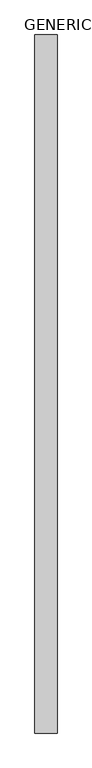
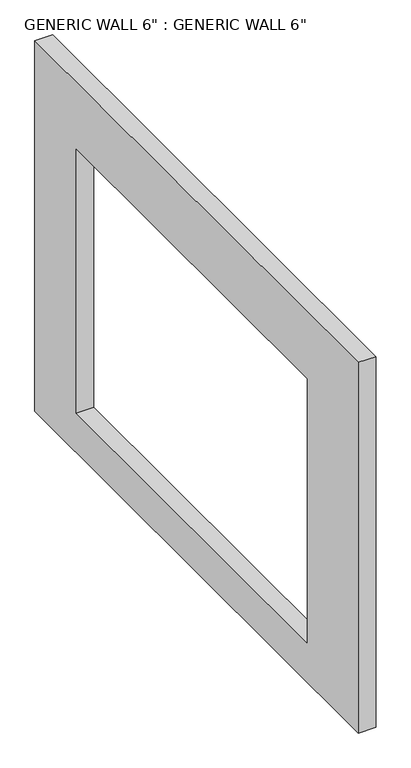
"""IFC4 building model written with IfcOpenShell, lengths in millimetres: proxy geometry."""

from ifc_helpers import new_model, si_unit, frame, origin, place, context, project, spatial, polyline, outline, extrude, source, transform, mapped, element, save


def proxy_c6281e4c(model_context):
    return source(origin(), model_context, "Body", "SweptSolid", [
        extrude(outline(polyline([(-13640.202305, 3352.8), (-8842.6396616, 3352.8), (-8842.6396616, 0.0), (-13640.202305, 0.0), (-13640.202305, 3352.8)]), holes=[polyline([(-12878.202305, 352.9993493), (-9452.2396616, 352.9993493), (-9452.2396616, 2743.2), (-12878.202305, 2743.2), (-12878.202305, 352.9993493)])]), frame((-11796.2293601, 0.0, 0.0), z_axis=(1.0, 0.0, 0.0), x_axis=(0.0, 1.0, 0.0)), (0.0, 0.0, 1.0), 152.4),
    ])


if __name__ == "__main__":
    model = new_model("IFC4")
    model_context = context("Model", 3, world=origin())
    ifc_project = project(units=[si_unit("LENGTHUNIT", "METRE", prefix="MILLI")], contexts=[model_context])
    site = spatial("IfcSite", under=ifc_project)
    building = spatial("IfcBuilding", under=site)
    placement = place(None, origin())
    proxy_shape = proxy_c6281e4c(model_context)
    element("IfcBuildingElementProxy", 1, Name="GENERIC WALL 6\" : GENERIC WALL 6\"", ObjectType="GENERIC WALL 6\" : GENERIC WALL 6\"", at=placement, inside=building, context=model_context, shape_type="MappedRepresentation", body=[
        mapped(proxy_shape, transform((0.0, 0.0, 0.0), x_axis=(1.0, 0.0, 0.0), y_axis=(0.0, 1.0, 0.0), z_axis=(0.0, 0.0, 1.0))),
    ])
    save(model, "model.ifc")

# Revit data of these elements
# Element 1 (IfcBuildingElementProxy, "GENERIC WALL 6\" : GENERIC WALL 6\"")
#   Materials on its faces: "ACCENT BEIGE COLOUR"
# Materials
#   "ACCENT BEIGE COLOUR": class "Generic", colour RGB 120 120 120, transparency 0, Cost = 0
